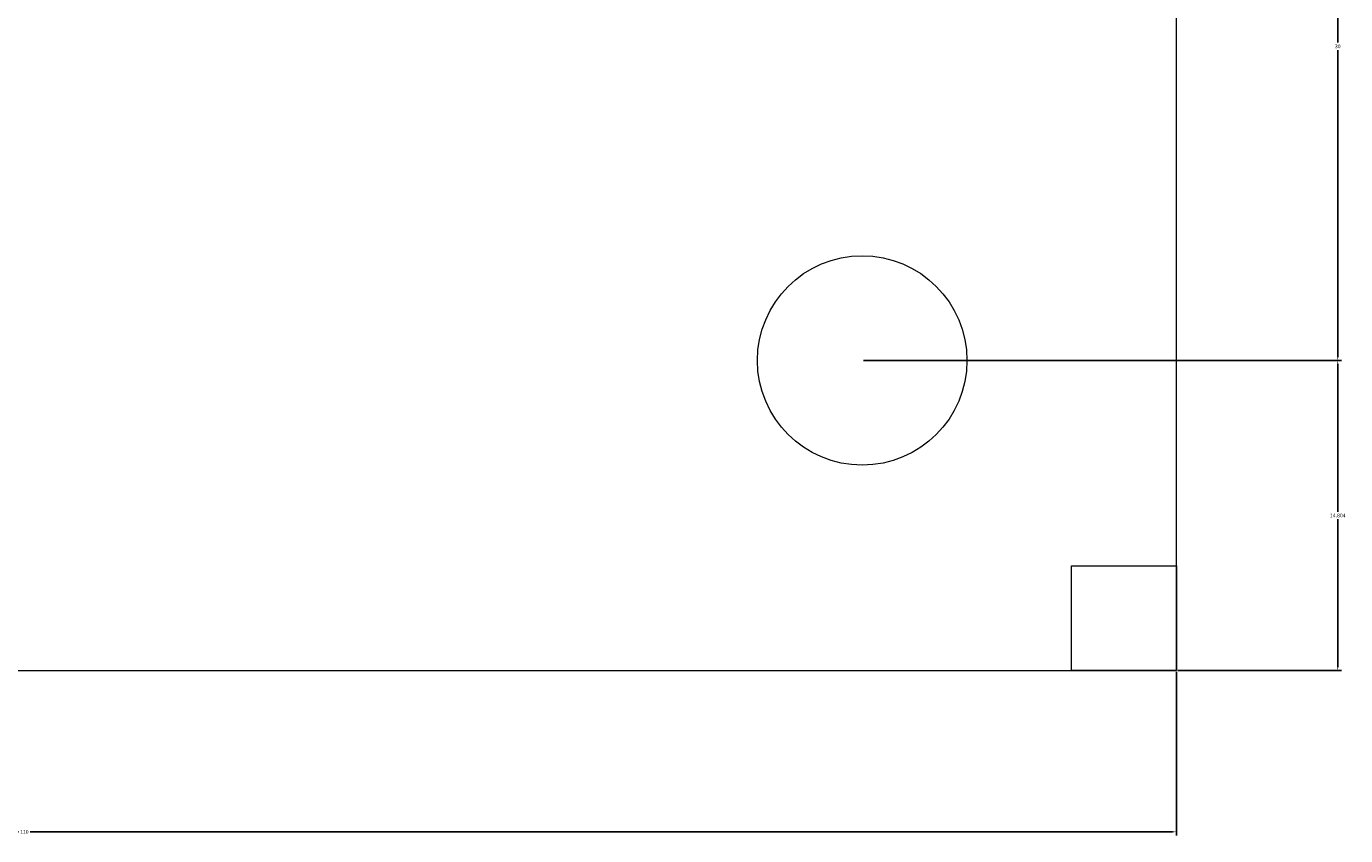
# Model space of a CAD drawing. Units: inches. Extents: x -19 to 107, y -27 to 49.
# Tile 3 of 4: x 44 to 107, y -27 to 12. Entities that reach past the tile are written whole.
import ezdxf

# ---------------------------------------------------------------- set-up
doc = ezdxf.new("R2010")
doc.units = ezdxf.units.IN
doc.header["$MEASUREMENT"] = 0
doc.layers.add('M-CONS', color=8, linetype='Continuous', lineweight=18)
doc.layers.add('M-DIMS', color=2, linetype='Continuous', lineweight=18)
doc.styles.get("Standard").update_dxf_attribs({"font": 'arial.ttf'})
doc.dimstyles.get("Standard").update_dxf_attribs({"dimtxt": 0.18, "dimasz": 0.18, "dimexe": 0.18, "dimexo": 0.0625, "dimgap": 0.09, "dimtad": 0, "dimtih": 1, "dimtoh": 1, "dimdec": 4, "dimzin": 0, "dimdsep": 46, "dimtxsty": 'Standard', "dimcen": 0.09, "dimadec": 0, "dimazin": 0, "dimtfac": 1, "dimtdec": 4, "dimtofl": 0, "dimtmove": 0, "dimatfit": 3, "dimfxl": 1, "dimtolj": 1, "dimtzin": 0, "dimarcsym": 0})

# ---------------------------------------------------------------- blocks, each defined once
blk = doc.blocks.new('*D1')
at = {"layer": 'Defpoints', "color": 0, "transparency": 16777216}
for p in [(-10.937, 10.82), (99.063, -19.18), (99.063, -26.885)]:
    blk.add_point(p, dxfattribs=at)
at = {"layer": 'M-DIMS', "color": 0, "lineweight": -2, "transparency": 16777216}
for p, q in [((-10.937, 10.758), (-10.937, -27.065)), ((99.063, -19.242), (99.063, -27.065)), ((-10.757, -26.885), (43.783, -26.885)), ((98.883, -26.885), (44.344, -26.885))]:
    blk.add_line(p, q, dxfattribs=at)
at = {"layer": 'M-DIMS', "color": 0, "transparency": 16777216}
for points in [[(-10.757, -26.855), (-10.757, -26.915), (-10.937, -26.885)], [(98.883, -26.855), (98.883, -26.915), (99.063, -26.885)]]:
    blk.add_solid(points, dxfattribs=at)
at = {"layer": 'M-DIMS', "color": 0, "transparency": 16777216, "insert": (44.063, -26.885), "char_height": 0.18, "attachment_point": 5}
blk.add_mtext('\\A1;110', dxfattribs=at)
blk = doc.blocks.new('*D7')
at = {"layer": 'Defpoints', "color": 0, "transparency": 16777216}
for p in [(84.063, 25.624), (106.768, 25.624), (84.063, -4.376)]:
    blk.add_point(p, dxfattribs=at)
at = {"layer": 'M-DIMS', "color": 0, "lineweight": -2, "transparency": 16777216}
for p, q in [((84.126, 25.624), (106.948, 25.624)), ((106.768, 25.444), (106.768, 10.806)), ((106.768, -4.196), (106.768, 10.443)), ((84.126, -4.376), (106.948, -4.376))]:
    blk.add_line(p, q, dxfattribs=at)
at = {"layer": 'M-DIMS', "color": 0, "transparency": 16777216}
for points in [[(106.738, 25.444), (106.798, 25.444), (106.768, 25.624)], [(106.738, -4.196), (106.798, -4.196), (106.768, -4.376)]]:
    blk.add_solid(points, dxfattribs=at)
at = {"layer": 'M-DIMS', "color": 0, "transparency": 16777216, "insert": (106.768, 10.624), "char_height": 0.18, "attachment_point": 5}
blk.add_mtext('\\A1;30', dxfattribs=at)
blk = doc.blocks.new('*D8')
at = {"layer": 'Defpoints', "color": 0, "transparency": 16777216}
for p in [(84.063, -4.376), (106.768, -4.376), (99.063, -19.18)]:
    blk.add_point(p, dxfattribs=at)
at = {"layer": 'M-DIMS', "color": 0, "lineweight": -2, "transparency": 16777216}
for p, q in [((84.126, -4.376), (106.948, -4.376)), ((106.768, -4.556), (106.768, -11.596)), ((106.768, -19), (106.768, -11.96)), ((99.126, -19.18), (106.948, -19.18))]:
    blk.add_line(p, q, dxfattribs=at)
at = {"layer": 'M-DIMS', "color": 0, "transparency": 16777216}
for points in [[(106.738, -4.556), (106.798, -4.556), (106.768, -4.376)], [(106.738, -19), (106.798, -19), (106.768, -19.18)]]:
    blk.add_solid(points, dxfattribs=at)
at = {"layer": 'M-DIMS', "color": 0, "transparency": 16777216, "insert": (106.768, -11.778), "char_height": 0.18, "attachment_point": 5}
blk.add_mtext('\\A1;14.804', dxfattribs=at)

msp = doc.modelspace()

# ---------------------------------------------------------------- linework, layer by layer
at = {"layer": 'M-CONS'}
for p, q in [((99.0635, -19.18), (99.0635, 40.82)), ((99.0635, -19.18), (99.0635, -4.18)), ((19.0635, -19.18), (99.0635, -19.18))]:
    msp.add_line(p, q, dxfattribs=at)
at = {"layer": 'M-CONS', "elevation": 20}
msp.add_lwpolyline([(99.0635, -19.18), (94.0635, -19.18), (94.0635, -14.18), (99.0635, -14.18)], close=True, dxfattribs=at)
at = {"layer": 'M-CONS'}
msp.add_circle((84.0635, -4.3755, 45), 5, dxfattribs=at)

# ---------------------------------------------------------------- dimensions: what is measured, and where the dimension line sits
at = {"layer": 'M-DIMS'}
for base, p1, p2, override, picture, middle in [((106.7685, 25.6245), (84.0635, -4.3755), (84.0635, 25.6245), {"dimdec": 0, "dimlfac": 1, "dimrnd": 0, "dimzin": 0, "dimdsep": 46, "dimlunit": 2}, '*D7', (106.7685, 10.6245)), ((106.7685, -4.37552), (99.0635, -19.17999), (84.0635, -4.37552), {"dimdec": 3, "dimlfac": 1, "dimrnd": 0, "dimzin": 0, "dimdsep": 46, "dimlunit": 2}, '*D8', (106.7685, -11.77775))]:
    dim = msp.add_linear_dim(base=base, p1=p1, p2=p2, angle=90, dimstyle='Standard', override=override, dxfattribs=at)
    dim.commit()
    dim.dimension.update_dxf_attribs({"geometry": picture, "text_midpoint": middle})
dim = msp.add_linear_dim(base=(99.0635, -26.885), p1=(-10.9365, 10.82), p2=(99.0635, -19.18), dimstyle='Standard', override={"dimdec": 0, "dimlfac": 1, "dimrnd": 0, "dimzin": 0, "dimdsep": 46, "dimlunit": 2}, dxfattribs=at)
dim.commit()
dim.dimension.update_dxf_attribs({"geometry": '*D1', "text_midpoint": (44.0635, -26.885)})

doc.saveas('drawing.dxf')
